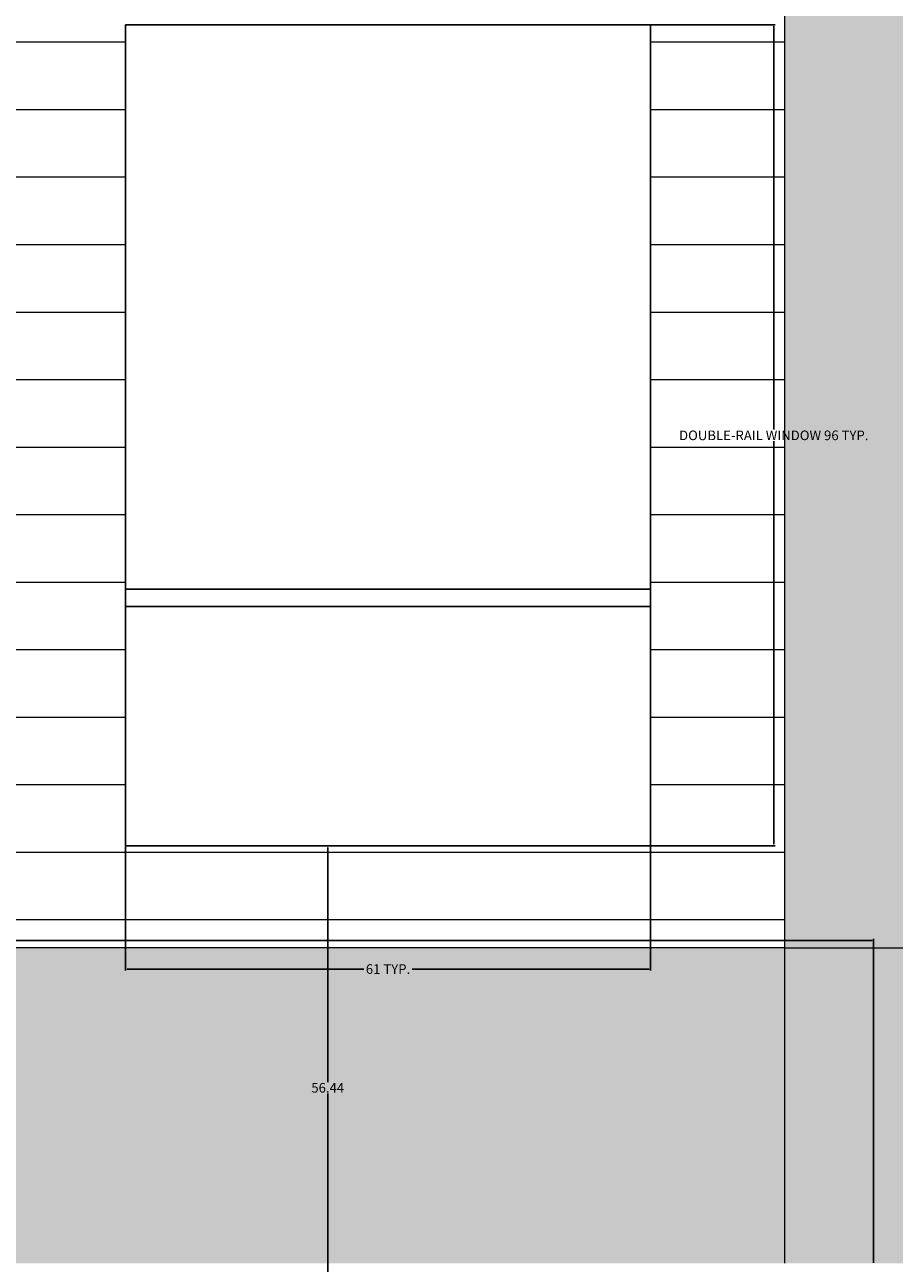
# Model space of a CAD drawing. Units: inches. Extents: x 8 to 634, y 41 to 867.
# Tile 4 of 21: x 196 to 297, y 236 to 380. Entities that reach past the tile are written whole.
import ezdxf

# ---------------------------------------------------------------- set-up
doc = ezdxf.new("R2010")
doc.units = ezdxf.units.IN
doc.header["$MEASUREMENT"] = 0
for name, color, linetype, lineweight in [('A-ANNO-DIMS', 2, 'Continuous', 18), ('A-GLAZ', 4, 'Continuous', 25), ('A-WALL-PANL', 7, 'Continuous', 18), ('A-WALL-PATT', 8, 'Continuous', 9)]:
    doc.layers.add(name, color=color, linetype=linetype, lineweight=lineweight)
doc.styles.get("Standard").update_dxf_attribs({"font": 'arial.ttf'})
doc.dimstyles.get("Standard").update_dxf_attribs({"dimtxt": 1.125, "dimasz": 0.18, "dimexe": 0.18, "dimexo": 0.0625, "dimgap": 0.09, "dimtad": 0, "dimtih": 1, "dimtoh": 1, "dimdec": 4, "dimzin": 0, "dimdsep": 46, "dimlunit": 4, "dimtxsty": 'Standard', "dimcen": 0.09, "dimadec": 0, "dimazin": 0, "dimtfac": 1, "dimtdec": 4, "dimtofl": 0, "dimtmove": 0, "dimatfit": 3, "dimfxl": 1, "dimtolj": 1, "dimtzin": 0, "dimarcsym": 0})

# ---------------------------------------------------------------- blocks, each defined once
blk = doc.blocks.new('WIN-DOUBLE-RAIL')
for p, q in [((0, 29.93), (61.23, 29.93)), ((0, 27.93), (61.23, 27.93))]:
    blk.add_line(p, q)
blk.add_lwpolyline([(0, 95.77), (61.23, 95.77), (61.23, 0), (0, 0)], close=True)
blk = doc.blocks.new('*D11')
at = {"layer": 'A-ANNO-DIMS', "color": 0, "lineweight": -2, "transparency": 16777216}
for p, q in [((269.05, 380.01), (283.53, 380.01)), ((283.35, 379.83), (283.35, 332.8)), ((283.35, 284.42), (283.35, 331.45)), ((269.05, 284.24), (283.53, 284.24))]:
    blk.add_line(p, q, dxfattribs=at)
at = {"layer": 'A-ANNO-DIMS', "color": 0, "transparency": 16777216}
for points in [[(283.32, 379.83), (283.38, 379.83), (283.35, 380.01)], [(283.32, 284.42), (283.38, 284.42), (283.35, 284.24)]]:
    blk.add_solid(points, dxfattribs=at)
at = {"layer": 'Defpoints', "color": 0, "transparency": 16777216}
for p in [(268.99, 380.01), (283.35, 380.01), (268.99, 284.24)]:
    blk.add_point(p, dxfattribs=at)
at = {"layer": 'A-ANNO-DIMS', "color": 0, "transparency": 16777216, "insert": (283.35, 332.12), "char_height": 1.125, "attachment_point": 5}
blk.add_mtext('\\A1;DOUBLE-RAIL WINDOW 96 TYP.', dxfattribs=at)
blk = doc.blocks.new('*D12')
at = {"layer": 'A-ANNO-DIMS', "color": 0, "lineweight": -2, "transparency": 16777216}
for p, q in [((207.75, 284.18), (207.75, 269.69)), ((268.99, 284.18), (268.99, 269.69)), ((207.93, 269.87), (235.54, 269.87)), ((268.81, 269.87), (241.2, 269.87))]:
    blk.add_line(p, q, dxfattribs=at)
at = {"layer": 'A-ANNO-DIMS', "color": 0, "transparency": 16777216}
for points in [[(207.93, 269.9), (207.93, 269.84), (207.75, 269.87)], [(268.81, 269.9), (268.81, 269.84), (268.99, 269.87)]]:
    blk.add_solid(points, dxfattribs=at)
at = {"layer": 'Defpoints', "color": 0, "transparency": 16777216}
for p in [(207.75, 284.24), (268.99, 284.24), (268.99, 269.87)]:
    blk.add_point(p, dxfattribs=at)
at = {"layer": 'A-ANNO-DIMS', "color": 0, "transparency": 16777216, "insert": (238.37, 269.87), "char_height": 1.125, "attachment_point": 5}
blk.add_mtext('\\A1;61 TYP.', dxfattribs=at)
blk = doc.blocks.new('*D42')
at = {"layer": 'A-ANNO-DIMS', "color": 0, "lineweight": -2, "transparency": 16777216}
for p, q in [((268.93, 284.24), (231.16, 284.23)), ((231.34, 284.05), (231.34, 256.68)), ((231.35, 227.98), (231.34, 255.35)), ((268.94, 227.8), (231.17, 227.8))]:
    blk.add_line(p, q, dxfattribs=at)
at = {"layer": 'A-ANNO-DIMS', "color": 0, "transparency": 16777216}
for points in [[(231.37, 284.05), (231.31, 284.05), (231.34, 284.23)], [(231.38, 227.98), (231.32, 227.98), (231.35, 227.8)]]:
    blk.add_solid(points, dxfattribs=at)
at = {"layer": 'Defpoints', "color": 0, "transparency": 16777216}
for p in [(231.34, 284.23), (268.99, 284.24), (269, 227.8)]:
    blk.add_point(p, dxfattribs=at)
at = {"layer": 'A-ANNO-DIMS', "color": 0, "transparency": 16777216, "insert": (231.34, 256.02), "char_height": 1.125, "attachment_point": 5}
blk.add_mtext('\\A1;56.44', dxfattribs=at)
blk = doc.blocks.new('*D65')
at = {"layer": 'A-ANNO-DIMS', "color": 0, "lineweight": -2, "transparency": 16777216}
for p, q in [((61.18, 235.62), (61.18, 273.39)), ((61.36, 273.21), (176.09, 273.21)), ((294.82, 273.21), (180.09, 273.21)), ((295, 235.62), (295, 273.39))]:
    blk.add_line(p, q, dxfattribs=at)
at = {"layer": 'A-ANNO-DIMS', "color": 0, "transparency": 16777216}
for points in [[(61.36, 273.24), (61.36, 273.18), (61.18, 273.21)], [(294.82, 273.24), (294.82, 273.18), (295, 273.21)]]:
    blk.add_solid(points, dxfattribs=at)
at = {"layer": 'Defpoints', "color": 0, "transparency": 16777216}
for p in [(295, 273.21), (61.18, 235.56), (295, 235.56)]:
    blk.add_point(p, dxfattribs=at)
at = {"layer": 'A-ANNO-DIMS', "color": 0, "transparency": 16777216, "insert": (178.09, 273.21), "char_height": 1.125, "attachment_point": 5}
blk.add_mtext('\\A1;233.8', dxfattribs=at)

msp = doc.modelspace()

# ---------------------------------------------------------------- hatches: boundary and pattern name
at = {"layer": 'A-WALL-PATT', "transparency": 33554687}
h = msp.add_hatch(dxfattribs=at)
h.set_pattern_fill('AR-CONC', color=256, scale=3.2)
h.paths.add_polyline_path([(119.7065, 697.6655), (47.3401, 697.6655), (47.3401, 569.1705), (119.7065, 569.1705)])
h.paths.add_polyline_path([(202.1558, 697.6655), (119.7065, 697.6655), (119.7065, 569.1705), (202.1558, 569.1705)])
h.paths.add_polyline_path([(284.6051, 697.6655), (202.1558, 697.6655), (202.1558, 569.1705), (284.6051, 569.1705)])
h.paths.add_polyline_path([(119.7065, 569.1705), (47.3401, 569.1705), (47.3401, 523.5555), (47.3401, 449.7533), (119.7065, 449.7533)])
h.paths.add_polyline_path([(342.6544, 682.1444), (360.785, 697.6655), (284.6051, 697.6655), (284.6051, 569.1705), (342.6544, 569.1705)])
h.paths.add_polyline_path([(342.6544, 569.1705), (284.6051, 569.1705), (284.6051, 449.7533), (342.6544, 449.7533)])
h.paths.add_polyline_path([(418.2881, 691.978), (418.2881, 697.6655), (360.785, 697.6655), (360.785, 569.1705), (418.2881, 569.1705)])
h.paths.add_polyline_path([(418.2881, 569.1705), (360.785, 569.1705), (360.785, 523.5555), (360.785, 449.7533), (418.2881, 449.7533)])
h.paths.add_polyline_path([(594.3501, 697.6655), (539.0002, 697.6655), (539.0002, 691.978), (539.0002, 569.1705), (594.3501, 569.1705)])
h.paths.add_polyline_path([(594.3501, 523.5555), (594.3501, 569.1705), (539.0002, 569.1705), (539.0002, 451.6305), (594.3501, 451.6305)])
h.paths.add_polyline_path([(594.3501, 451.6305), (539.0002, 451.6305), (539.0002, 391.7598), (594.3501, 391.7598)])
h.paths.add_polyline_path([(594.3501, 391.7598), (539.0002, 391.7598), (539.0002, 276.166), (594.3501, 276.166)])
h.paths.add_polyline_path([(418.2881, 449.7533), (360.785, 449.7533), (360.785, 391.7598), (418.2881, 391.7598)])
h.paths.add_polyline_path([(342.6544, 449.7533), (284.6051, 449.7533), (284.6051, 391.7598), (342.6544, 391.7598)])
h.paths.add_polyline_path([(342.6544, 391.7598), (284.6051, 391.7598), (284.6051, 272.3426), (342.6544, 272.3426)])
h.paths.add_polyline_path([(418.2881, 391.7598), (360.785, 391.7598), (360.785, 272.3426), (418.2881, 272.3426)])
h.paths.add_polyline_path([(418.2881, 272.3426), (360.785, 272.3426), (360.785, 235.5555), (418.2881, 235.5555)])
h.paths.add_polyline_path([(342.6544, 272.3426), (284.6051, 272.3426), (284.6051, 235.5555), (295.0049, 235.5555), (342.6544, 235.5555)])
h.paths.add_polyline_path([(594.3501, 276.166), (539.0002, 276.166), (539.0002, 228.4951), (594.3501, 228.4951)])
h.paths.add_polyline_path([(594.3501, 228.4951), (539.0002, 228.4951), (539.0002, 91.5417), (594.3501, 91.5417)])
h.paths.add_polyline_path([(418.2881, 235.5555), (360.785, 235.5555), (360.785, 91.5417), (418.2881, 91.5417)])
h.paths.add_polyline_path([(284.6051, 272.3426), (119.7065, 272.3426), (119.7065, 235.5555), (284.6051, 235.5555)])
h.paths.add_polyline_path([(119.7065, 272.3426), (47.3401, 272.3426), (47.3401, 235.5555), (47.3401, 91.5555), (63.5448, 91.5555), (63.5448, 227.8036), (268.998, 227.8036), (268.998, 91.5555), (295.0049, 91.5555), (295.0049, 222.583), (271.9787, 222.583), (271.9787, 229.0481), (62.4019, 229.0481), (62.4019, 222.583), (61.1827, 222.583), (61.1827, 235.5555), (119.7065, 235.5555)])
h.paths.add_polyline_path([(119.7065, 391.7598), (47.3401, 391.7598), (47.3401, 379.5555), (47.3401, 272.3426), (119.7065, 272.3426)])
h.paths.add_polyline_path([(119.7065, 449.7533), (47.3401, 449.7533), (47.3401, 391.7598), (119.7065, 391.7598)])
h.paths.add_polyline_path([(202.1558, 449.7533), (119.7065, 449.7533), (119.7065, 391.7598), (202.1558, 391.7598)])
h.paths.add_polyline_path([(284.6051, 449.7533), (202.1558, 449.7533), (202.1558, 391.7598), (284.6051, 391.7598)])
at = {"layer": 'A-WALL-PATT', "transparency": 33554681}
h = msp.add_hatch(dxfattribs=at)
h.set_pattern_fill('ANSI31', color=256, scale=63, angle=135)
h.paths.add_polyline_path([(284.6051, 391.7598), (119.7065, 391.7598), (119.7065, 272.3426), (284.6051, 272.3426)])
h.paths.add_polyline_path([(193.1116, 284.2398), (131.8771, 284.2398), (131.8771, 380.0085), (193.1116, 380.0085)], flags=16)
h.paths.add_polyline_path([(207.7547, 380.0085), (268.9893, 380.0085), (268.9893, 284.2398), (207.7547, 284.2398)], flags=16)
h.paths.add_polyline_path([(342.6544, 235.5555), (295.0049, 235.5555), (295.0049, 91.5417), (342.6544, 91.5417)])

# ---------------------------------------------------------------- linework, layer by layer
at = {"layer": 'A-WALL-PANL'}
for q in [(418.2881, 272.3426), (284.6051, 235.5555)]:
    msp.add_line((284.6051, 272.3426), q, dxfattribs=at)
msp.add_lwpolyline([(119.7065, 391.7598), (284.6051, 391.7598), (284.6051, 272.3426), (119.7065, 272.3426)], close=True, dxfattribs=at)

# ---------------------------------------------------------------- block references
at = {"layer": 'A-GLAZ'}
msp.add_blockref('WIN-DOUBLE-RAIL', (207.7546, 284.24), dxfattribs=at)

# ---------------------------------------------------------------- dimensions: what is measured, and where the dimension line sits
at = {"layer": 'A-ANNO-DIMS'}
dim = msp.add_linear_dim(base=(283.3546, 380.0085), p1=(268.9893, 284.2398), p2=(268.9893, 380.0085), angle=90, text='DOUBLE-RAIL WINDOW <> TYP.', dimstyle='Standard', override={"dimdec": 0, "dimlfac": 1, "dimrnd": 0, "dimzin": 0, "dimdsep": 46, "dimlunit": 2}, dxfattribs=at)
dim.commit()
dim.dimension.update_dxf_attribs({"geometry": '*D11', "text_midpoint": (283.3546, 332.1241)})
dim = msp.add_linear_dim(base=(268.9893, 269.8745), p1=(207.7547, 284.2398), p2=(268.9893, 284.2398), text='<> TYP.', dimstyle='Standard', override={"dimdec": 0, "dimlfac": 1, "dimrnd": 0, "dimzin": 0, "dimdsep": 46, "dimlunit": 2}, dxfattribs=at)
dim.commit()
dim.dimension.update_dxf_attribs({"geometry": '*D12', "text_midpoint": (238.372, 269.8745)})
dim = msp.add_linear_dim(base=(231.3393, 284.234), p1=(268.998, 227.8036), p2=(268.9893, 284.2398), angle=90.00885, dimstyle='Standard', override={"dimdec": 2, "dimlfac": 1, "dimrnd": 0, "dimzin": 0, "dimdsep": 46, "dimlunit": 2}, dxfattribs=at)
dim.commit()
dim.dimension.update_dxf_attribs({"geometry": '*D42', "text_midpoint": (231.3436, 256.0159)})
dim = msp.add_linear_dim(base=(295.0049, 273.2055), p1=(61.1827, 235.5555), p2=(295.0049, 235.5555), dimstyle='Standard', override={"dimdec": 1, "dimlfac": 1, "dimrnd": 0, "dimzin": 0, "dimdsep": 46, "dimlunit": 2}, dxfattribs=at)
dim.commit()
dim.dimension.update_dxf_attribs({"geometry": '*D65', "text_midpoint": (178.0938, 273.2055)})

doc.saveas('drawing.dxf')
